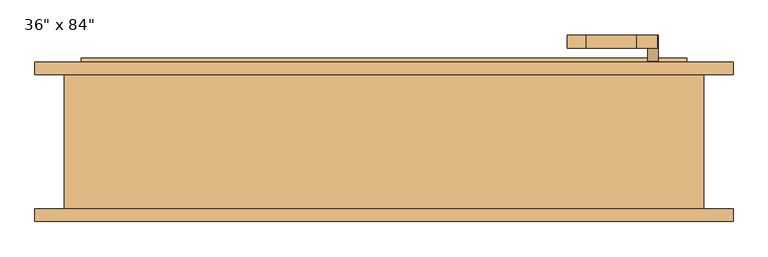
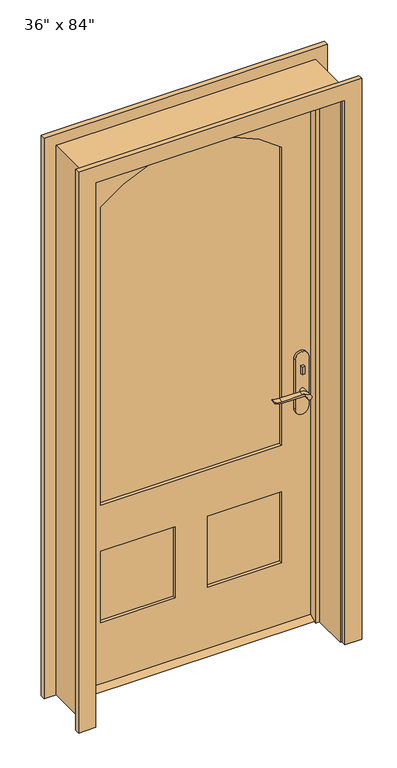
"""IFC4 building model written with IfcOpenShell, lengths in millimetres: door geometry."""

from ifc_helpers import new_model, si_unit, point, frame, frame_2d, origin, place, context, project, spatial, polyline, circle_curve, trimmed, segment, composite_curve, outline, extrude, faceted_brep, source, transform, mapped, element, save


def door_4a215221(model_context):
    return source(origin(), model_context, "Body", "SolidModel", [
        extrude(outline(polyline([(63.5, 12.7), (98.425, 12.7), (123.825, 0.0), (38.1, 0.0), (63.5, 12.7)])), frame((-457.2, 0.0, 0.0), z_axis=(1.0, 0.0, 0.0), x_axis=(0.0, 1.0, 0.0)), (0.0, 0.0, 1.0), 914.4),
        extrude(outline(polyline([(411.4, 43.5), (401.4, 43.5), (401.4, 53.5), (411.4, 53.5), (411.4, 43.5)])), frame((0.0, 0.0, 981.9), z_axis=(0.0, 0.0, 1.0), x_axis=(1.0, 0.0, 0.0)), (0.0, 0.0, 1.0), 30.0),
        extrude(outline(composite_curve([segment(trimmed(circle_curve(frame_2d((996.9, 406.4)), 8.0), [point((996.9, 398.4))], [point((996.9, 414.4))], False, "CARTESIAN"), True, "CONTINUOUS"), segment(trimmed(circle_curve(frame_2d((996.9, 406.4)), 8.0), [point((996.9, 414.4))], [point((996.9, 398.4))], False, "CARTESIAN"), True, "CONTINUOUS")], self_intersect=False)), frame((0.0, 108.425, 0.0), z_axis=(0.0, 1.0, 0.0), x_axis=(0.0, 0.0, 1.0)), (0.0, 0.0, 1.0), 10.0),
        extrude(outline(composite_curve([segment(trimmed(circle_curve(frame_2d((897.1555521, 382.7324871)), 37.2832219), [point((919.0523287, 412.9081363))], [point((934.4, 381.0325667))], False, "CARTESIAN"), True, "CONTINUOUS"), segment(polyline([(934.4, 381.0325667), (934.4, 304.7564091)]), True, "CONTINUOUS"), segment(trimmed(circle_curve(frame_2d((1017.6850638, 304.8227909)), 83.2850902), [point((934.4, 304.7564091))], [point((939.4, 276.4))], True, "CARTESIAN"), True, "CONTINUOUS"), segment(polyline([(939.4, 276.4), (936.6135558, 276.4)]), True, "CONTINUOUS"), segment(trimmed(circle_curve(frame_2d((986.6709207, 308.3396612)), 59.3791355), [point((936.6135558, 276.4))], [point((927.4, 304.7564091))], False, "CARTESIAN"), True, "CONTINUOUS"), segment(polyline([(927.4, 304.7564091), (927.4, 381.0138099)]), True, "CONTINUOUS"), segment(trimmed(circle_curve(frame_2d((909.2738613, 381.0138099)), 18.1261387), [point((927.4, 381.0138099))], [point((914.4, 398.4))], True, "CARTESIAN"), True, "CONTINUOUS"), segment(trimmed(circle_curve(frame_2d((914.4, 406.4)), 8.0), [point((914.4, 398.4))], [point((919.0523287, 412.9081363))], False, "CARTESIAN"), True, "CONTINUOUS")], self_intersect=False)), frame((0.0, 3.5, 0.0), z_axis=(0.0, 1.0, 0.0), x_axis=(0.0, 0.0, 1.0)), (0.0, 0.0, 1.0), 20.0),
        extrude(outline(composite_curve([segment(trimmed(circle_curve(frame_2d((914.4, 406.4)), 8.0), [point((914.3999903, 398.4))], [point((919.0523287, 412.9081363))], False, "CARTESIAN"), True, "CONTINUOUS"), segment(trimmed(circle_curve(frame_2d((897.1555521, 382.7324871)), 37.2832219), [point((919.0523287, 412.9081363))], [point((934.4, 381.0325667))], False, "CARTESIAN"), True, "CONTINUOUS"), segment(polyline([(934.4, 381.0325667), (934.4, 304.7564091)]), True, "CONTINUOUS"), segment(trimmed(circle_curve(frame_2d((1017.6850638, 304.8227909)), 83.2850902), [point((934.4, 304.7564091))], [point((939.4, 276.4))], True, "CARTESIAN"), True, "CONTINUOUS"), segment(polyline([(939.4, 276.4), (936.6135558, 276.4)]), True, "CONTINUOUS"), segment(trimmed(circle_curve(frame_2d((986.6709207, 308.3396612)), 59.3791355), [point((936.6135558, 276.4))], [point((927.4, 304.7564091))], False, "CARTESIAN"), True, "CONTINUOUS"), segment(polyline([(927.4, 304.7564091), (927.4, 381.0138122)]), True, "CONTINUOUS"), segment(trimmed(circle_curve(frame_2d((909.2738682, 381.0138122)), 18.1261318), [point((927.4, 381.0138122))], [point((914.3999903, 398.4))], True, "CARTESIAN"), True, "CONTINUOUS")], self_intersect=False)), frame((0.0, 138.425, 0.0), z_axis=(0.0, 1.0, 0.0), x_axis=(0.0, 0.0, 1.0)), (0.0, 0.0, 1.0), 20.0),
        extrude(outline(composite_curve([segment(trimmed(circle_curve(frame_2d((914.4, 406.4)), 8.0), [point((914.4, 398.4))], [point((914.4, 414.4))], False, "CARTESIAN"), True, "CONTINUOUS"), segment(trimmed(circle_curve(frame_2d((914.4, 406.4)), 8.0), [point((914.4, 414.4))], [point((914.4, 398.4))], False, "CARTESIAN"), True, "CONTINUOUS")], self_intersect=False)), frame((0.0, 23.5, 0.0), z_axis=(0.0, 1.0, 0.0), x_axis=(0.0, 0.0, 1.0)), (0.0, 0.0, 1.0), 30.0),
        extrude(outline(composite_curve([segment(trimmed(circle_curve(frame_2d((914.4, 406.4)), 8.0), [point((914.4, 398.4))], [point((914.4, 414.4))], False, "CARTESIAN"), True, "CONTINUOUS"), segment(trimmed(circle_curve(frame_2d((914.4, 406.4)), 8.0), [point((914.4, 414.4))], [point((914.4, 398.4))], False, "CARTESIAN"), True, "CONTINUOUS")], self_intersect=False)), frame((0.0, 108.425, 0.0), z_axis=(0.0, 1.0, 0.0), x_axis=(0.0, 0.0, 1.0)), (0.0, 0.0, 1.0), 30.0),
        extrude(outline(composite_curve([segment(polyline([(844.4, 431.4), (1039.4, 431.4)]), True, "CONTINUOUS"), segment(trimmed(circle_curve(frame_2d((1039.4, 406.4)), 25.0), [point((1039.4, 431.4))], [point((1039.4, 381.4))], False, "CARTESIAN"), True, "CONTINUOUS"), segment(polyline([(1039.4, 381.4), (844.4, 381.4)]), True, "CONTINUOUS"), segment(trimmed(circle_curve(frame_2d((844.4, 406.4)), 25.0), [point((844.4, 381.4))], [point((844.4, 431.4))], False, "CARTESIAN"), True, "CONTINUOUS")], self_intersect=False)), frame((0.0, 53.5, 0.0), z_axis=(0.0, 1.0, 0.0), x_axis=(0.0, 0.0, 1.0)), (0.0, 0.0, 1.0), 10.0),
        extrude(outline(composite_curve([segment(polyline([(844.4, 431.4), (1039.4, 431.4)]), True, "CONTINUOUS"), segment(trimmed(circle_curve(frame_2d((1039.4, 406.4)), 25.0), [point((1039.4, 431.4))], [point((1039.4, 381.4))], False, "CARTESIAN"), True, "CONTINUOUS"), segment(polyline([(1039.4, 381.4), (844.4, 381.4)]), True, "CONTINUOUS"), segment(trimmed(circle_curve(frame_2d((844.4, 406.4)), 25.0), [point((844.4, 381.4))], [point((844.4, 431.4))], False, "CARTESIAN"), True, "CONTINUOUS")], self_intersect=False)), frame((0.0, 98.425, 0.0), z_axis=(0.0, 1.0, 0.0), x_axis=(0.0, 0.0, 1.0)), (0.0, 0.0, 1.0), 10.0),
        extrude(outline(polyline([(2133.6, -457.2), (12.7, -457.2), (12.7, 457.2), (2133.6, 457.2), (2133.6, -457.2)]), holes=[composite_curve([segment(polyline([(714.375, -336.55), (1885.95, -336.55)]), True, "CONTINUOUS"), segment(trimmed(circle_curve(frame_2d((1503.52125, 0.0)), 509.42875), [point((1885.95, -336.55))], [point((1885.95, 336.55))], True, "CARTESIAN"), True, "CONTINUOUS"), segment(polyline([(1885.95, 336.55), (714.375, 336.55), (714.375, -336.55)]), True, "CONTINUOUS")], self_intersect=False), polyline([(533.4, -60.325), (254.0, -60.325), (254.0, -336.55), (533.4, -336.55), (533.4, -60.325)]), polyline([(533.4, 336.55), (254.0, 336.55), (254.0, 60.325), (533.4, 60.325), (533.4, 336.55)])]), frame((0.0, 63.5, 0.0), z_axis=(0.0, 1.0, 0.0), x_axis=(0.0, 0.0, 1.0)), (0.0, 0.0, 1.0), 34.925),
        faceted_brep([(482.6, 98.425, 0.0), (482.6, -104.775, 0.0), (457.2, -104.775, 0.0), (457.2, 28.575, 0.0), (444.5, 28.575, 0.0), (444.5, 63.5, 0.0), (457.2, 63.5, 0.0), (457.2, 98.425, 0.0), (482.6, 98.425, 2159.0), (482.6, -104.775, 2159.0), (-482.6, -104.775, 2159.0), (-482.6, -104.775, 0.0), (-457.2, -104.775, 0.0), (-457.2, -104.775, 2133.6), (457.2, -104.775, 2133.6), (457.2, 28.575, 2133.6), (-457.2, 28.575, 2133.6), (-457.2, 28.575, 0.0), (-444.5, 28.575, 0.0), (-444.5, 28.575, 2120.9), (444.5, 28.575, 2120.9), (444.5, 63.5, 2120.9), (-444.5, 63.5, 2120.9), (-444.5, 63.5, 0.0), (-457.2, 63.5, 0.0), (-457.2, 63.5, 2133.6), (457.2, 63.5, 2133.6), (457.2, 98.425, 2133.6), (-457.2, 98.425, 2133.6), (-457.2, 98.425, 0.0), (-482.6, 98.425, 0.0), (-482.6, 98.425, 2159.0)], [[[0, 1, 2, 3, 4, 5, 6, 7]], [[1, 0, 8, 9]], [[2, 1, 9, 10, 11, 12, 13, 14]], [[3, 2, 14, 15]], [[4, 3, 15, 16, 17, 18, 19, 20]], [[5, 4, 20, 21]], [[6, 5, 21, 22, 23, 24, 25, 26]], [[7, 6, 26, 27]], [[0, 7, 27, 28, 29, 30, 31, 8]], [[9, 8, 31, 10]], [[15, 14, 13, 16]], [[21, 20, 19, 22]], [[27, 26, 25, 28]], [[30, 29, 24, 23, 18, 17, 12, 11]], [[10, 31, 30, 11]], [[16, 13, 12, 17]], [[22, 19, 18, 23]], [[28, 25, 24, 29]]]),
        extrude(outline(polyline([(-60.325, 75.1416667), (-336.55, 75.1416667), (-336.55, 86.7833333), (-60.325, 86.7833333), (-60.325, 75.1416667)])), frame((0.0, 0.0, 254.0), z_axis=(0.0, 0.0, 1.0), x_axis=(1.0, 0.0, 0.0)), (0.0, 0.0, 1.0), 279.4),
        extrude(outline(polyline([(336.55, 75.1416667), (60.325, 75.1416667), (60.325, 86.7833333), (336.55, 86.7833333), (336.55, 75.1416667)])), frame((0.0, 0.0, 254.0), z_axis=(0.0, 0.0, 1.0), x_axis=(1.0, 0.0, 0.0)), (0.0, 0.0, 1.0), 279.4),
        extrude(outline(composite_curve([segment(polyline([(714.375, -336.55), (714.375, 336.55), (1885.95, 336.55)]), True, "CONTINUOUS"), segment(trimmed(circle_curve(frame_2d((1503.52125, 0.0)), 509.42875), [point((1885.95, 336.55))], [point((1885.95, -336.55))], False, "CARTESIAN"), True, "CONTINUOUS"), segment(polyline([(1885.95, -336.55), (714.375, -336.55)]), True, "CONTINUOUS")], self_intersect=False)), frame((0.0, 77.47, 0.0), z_axis=(0.0, 1.0, 0.0), x_axis=(0.0, 0.0, 1.0)), (0.0, 0.0, 1.0), 6.985),
        extrude(outline(polyline([(0.0, -527.05), (0.0, -463.55), (2139.95, -463.55), (2139.95, 463.55), (0.0, 463.55), (0.0, 527.05), (2203.45, 527.05), (2203.45, -527.05), (0.0, -527.05)])), frame((0.0, -123.825, 0.0), z_axis=(0.0, 1.0, 0.0), x_axis=(0.0, 0.0, 1.0)), (0.0, 0.0, 1.0), 19.05),
        extrude(outline(polyline([(0.0, -527.05), (0.0, -463.55), (2139.95, -463.55), (2139.95, 463.55), (0.0, 463.55), (0.0, 527.05), (2203.45, 527.05), (2203.45, -527.05), (0.0, -527.05)])), frame((0.0, 98.425, 0.0), z_axis=(0.0, 1.0, 0.0), x_axis=(0.0, 0.0, 1.0)), (0.0, 0.0, 1.0), 19.05),
    ])


if __name__ == "__main__":
    model = new_model("IFC4")
    model_context = context("Model", 3, world=origin())
    ifc_project = project(units=[si_unit("LENGTHUNIT", "METRE", prefix="MILLI")], contexts=[model_context])
    site = spatial("IfcSite", under=ifc_project)
    building = spatial("IfcBuilding", under=site)
    placement = place(None, origin())
    door_shape = door_4a215221(model_context)
    element("IfcDoor", 1, ObjectType="36\" x 84\"", at=placement, inside=building, context=model_context, shape_type="MappedRepresentation", body=[
        mapped(door_shape, transform((0.0, 0.0, 0.0), x_axis=(1.0, 0.0, 0.0), y_axis=(0.0, 1.0, 0.0), z_axis=(0.0, 0.0, 1.0))),
    ])
    save(model, "model.ifc")

# Revit data of these elements
# Type "36\" x 84\""
#   Type Mark = "11"
#   Assembly Code = "B2030100"
#   Analytic Construction = "French door, wood frame with single glass"
#   Threshold Offset [instance default] = 0' - 0 1/2"
#   Thickness = 0' - 1 3/8"
#   Thermal Resistance (R) = 1.0696 (h·ft²·°F)/BTU
#   Swing Angle [instance default] = 90.00°
#   Stiles = 0' - 4 3/4"
#   Rough Width = 3' - 2"
#   Rough Height = 7' - 1"
#   Radius = 1' - 8.05625"
#   Lock Rail = 0' - 7 1/8"
#   Height = 7' - 0"
#   Width = 3' - 0"
#   Heat Transfer Coefficient (U) = 0.9350 BTU/(h·ft²·°F)
#   Door Offset [instance default] = 0' - 0"
#   Bottom Rail = 0' - 9 1/2"
#   Threshold [instance default] = yes
#   Function = 1
#   Exterior Trim [instance default] = yes
#   Trim Material = Cherry
#   Threshold Material = Cherry
#   Panel Material = Cherry
#   Glazing = Glass
#   Frame Material = Cherry
#   Door Handle Material = Aluminum
#   Visual Light Transmittance = 0
#   Solar Heat Gain Coefficient = 0
#   Wall Closure = (empty or 0)
#   Construction Type = (empty or 0)
# Element 1 (IfcDoor, "36\" x 84\"")
#   Materials on its faces: "Cherry", "Aluminum", "Glass"
# Materials
#   "Cherry": class "Wood", colour RGB 226 177 128, transparency 0, Description = "Prunus Serotina", Cost = 0
#   "Glass": class "Glass", colour RGB 0 128 192, transparency 0.75, Description = "Soda Lime Glass", Cost = 0
#   "Aluminum": class "Metal", colour RGB 247 247 247, transparency 0, Description = "Aluminum 6061", Cost = 0
